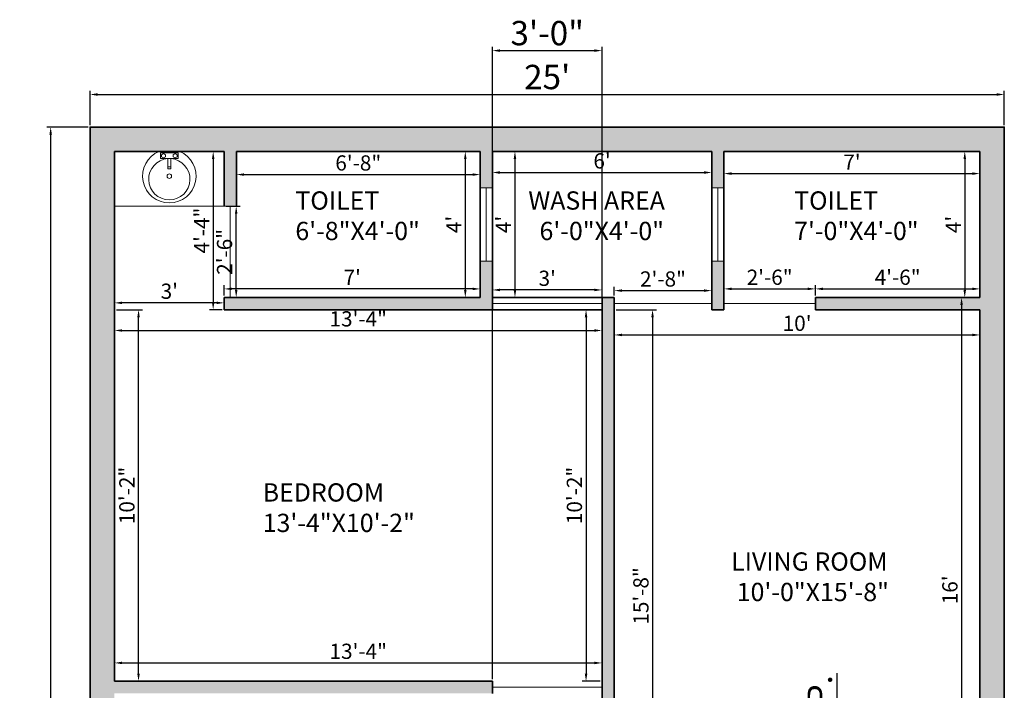
# Model space of a CAD drawing. Units: inches. Extents: x 3259 to 4981, y 1402 to 2026.
# Tile 9 of 11: x 4265 to 4588, y 1722 to 1942. Entities that reach past the tile are written whole.
import ezdxf

# ---------------------------------------------------------------- set-up
doc = ezdxf.new("R2010")
doc.units = ezdxf.units.IN
for name, color, linetype, lineweight in [('A-ANNO-DIMS', 2, 'Continuous', 13), ('A-AREA-IDEN', 7, 'Continuous', 18), ('A-DOOR', 3, 'Continuous', 18), ('A-FLOR-CASE', 8, 'Continuous', 18), ('A-FLOR-FIXT', 9, 'Continuous', 18), ('A-GLAZ', 4, 'Continuous', 18), ('A-WALL', 7, 'Continuous', 35), ('A-WALL-PATT', 252, 'Continuous', 13)]:
    doc.layers.add(name, color=color, linetype=linetype, lineweight=lineweight)
doc.styles.get("Standard").update_dxf_attribs({"font": 'arial.ttf'})
doc.dimstyles.new('ISO-25', dxfattribs={"dimtxt": 8, "dimasz": 2.5, "dimexe": 1.25, "dimexo": 0.625, "dimtad": 1, "dimdec": 1, "dimlunit": 3, "dimtxsty": 'Standard', "dimcen": 2.5, "dimclrd": 4, "dimclre": 4, "dimclrt": 1, "dimadec": 0, "dimazin": 0, "dimtfac": 1, "dimtdec": 1, "dimtmove": 0, "dimatfit": 3, "dimfxl": 1, "dimarcsym": 0})

# ---------------------------------------------------------------- blocks, each defined once
blk = doc.blocks.new('M_BATH_BASIN_Basin - Oval_P')
at = {"color": 0, "linetype": 'ByBlock', "lineweight": -2}
blk.add_lwpolyline([(0, 89.5, -5.027337), (0, -89.5)], format="xyb", close=True, dxfattribs=at)
blk.add_lwpolyline([(63.2, 12, -30), (63.2, -12, -1.097889)], format="xyb", dxfattribs=at)
for points in [[(13.2, -76.2), (13.2, 76.2), (63.2, 76.2), (63.2, -76.2)], [(19.1, 50.8), (28.7, 67.3), (47.7, 67.3), (57.2, 50.8), (47.7, 34.3), (28.7, 34.3)]]:
    blk.add_lwpolyline(points, close=True, dxfattribs=at)
for points in [[(63.2, 12), (151.6, 12), (151.6, -12), (63.2, -12)], [(134.3, 12), (134.3, -12)], [(28.7, -34.3), (47.7, -34.3), (57.2, -50.8), (47.7, -67.3), (28.7, -67.3), (19.1, -50.8), (28.7, -34.3)]]:
    blk.add_lwpolyline(points, dxfattribs=at)
blk.add_circle((216.2, 0), 20.1, dxfattribs=at)
at = {"layer": 'Defpoints'}
for p in [(0, 234), (0, -234)]:
    blk.add_point(p, dxfattribs=at)
blk = doc.blocks.new('*D83')
at = {"layer": 'A-ANNO-DIMS', "color": 0, "lineweight": -2, "transparency": 16777216}
for p, q in [((4288.33, 1907.74), (4288.33, 1919.06)), ((4290.83, 1917.81), (4585.83, 1917.81)), ((4588.33, 1907.74), (4588.33, 1919.06))]:
    blk.add_line(p, q, dxfattribs=at)
at = {"layer": 'A-ANNO-DIMS', "color": 0, "transparency": 16777216}
for points in [[(4290.83, 1918.23), (4290.83, 1917.39), (4288.33, 1917.81)], [(4585.83, 1918.23), (4585.83, 1917.39), (4588.33, 1917.81)]]:
    blk.add_solid(points, dxfattribs=at)
at = {"layer": 'Defpoints', "color": 0, "transparency": 16777216}
for p in [(4588.33, 1917.81), (4288.33, 1907.12), (4588.33, 1907.12)]:
    blk.add_point(p, dxfattribs=at)
at = {"layer": 'A-ANNO-DIMS', "color": 0, "transparency": 16777216, "insert": (4438.33, 1922.52), "char_height": 8, "attachment_point": 5}
blk.add_mtext("25'", dxfattribs=at)
blk = doc.blocks.new('*D84')
at = {"layer": 'A-ANNO-DIMS', "color": 0, "lineweight": -2, "transparency": 16777216}
for p, q in [((4287.71, 1907.12), (4274.14, 1907.12)), ((4275.39, 1904.62), (4275.39, 1477.62)), ((4287.71, 1475.12), (4274.14, 1475.12))]:
    blk.add_line(p, q, dxfattribs=at)
at = {"layer": 'A-ANNO-DIMS', "color": 0, "transparency": 16777216}
for points in [[(4274.97, 1904.62), (4275.81, 1904.62), (4275.39, 1907.12)], [(4274.97, 1477.62), (4275.81, 1477.62), (4275.39, 1475.12)]]:
    blk.add_solid(points, dxfattribs=at)
at = {"layer": 'Defpoints', "color": 0, "transparency": 16777216}
for p in [(4288.33, 1907.12), (4275.39, 1475.12), (4288.33, 1475.12)]:
    blk.add_point(p, dxfattribs=at)
at = {"layer": 'A-ANNO-DIMS', "color": 0, "transparency": 16777216, "insert": (4270.68, 1691.12), "char_height": 8, "attachment_point": 5, "rotation": 90}
blk.add_mtext("36'", dxfattribs=at)
blk = doc.blocks.new('*D79')
at = {"layer": 'A-ANNO-DIMS', "color": 0, "lineweight": -2, "transparency": 16777216}
for p, q in [((4580.33, 1846.49), (4580.33, 1837.58)), ((4460.33, 1843.37), (4460.33, 1837.58)), ((4462.83, 1838.83), (4577.83, 1838.83))]:
    blk.add_line(p, q, dxfattribs=at)
at = {"layer": 'A-ANNO-DIMS', "color": 0, "transparency": 16777216}
for points in [[(4462.83, 1839.25), (4462.83, 1838.42), (4460.33, 1838.83)], [(4577.83, 1839.25), (4577.83, 1838.42), (4580.33, 1838.83)]]:
    blk.add_solid(points, dxfattribs=at)
at = {"layer": 'Defpoints', "color": 0, "transparency": 16777216}
for p in [(4580.33, 1847.12), (4460.33, 1844), (4580.33, 1838.83)]:
    blk.add_point(p, dxfattribs=at)
at = {"layer": 'A-ANNO-DIMS', "color": 0, "transparency": 16777216, "insert": (4520.33, 1842.01), "char_height": 5, "attachment_point": 5}
blk.add_mtext("10'", dxfattribs=at)
blk = doc.blocks.new('*D80')
at = {"layer": 'A-ANNO-DIMS', "color": 0, "lineweight": -2, "transparency": 16777216}
for p, q in [((4460.96, 1847.12), (4474.15, 1847.12)), ((4472.9, 1844.62), (4472.9, 1661.62)), ((4460.96, 1659.12), (4474.15, 1659.12))]:
    blk.add_line(p, q, dxfattribs=at)
at = {"layer": 'A-ANNO-DIMS', "color": 0, "transparency": 16777216}
for points in [[(4472.49, 1844.62), (4473.32, 1844.62), (4472.9, 1847.12)], [(4472.49, 1661.62), (4473.32, 1661.62), (4472.9, 1659.12)]]:
    blk.add_solid(points, dxfattribs=at)
at = {"layer": 'Defpoints', "color": 0, "transparency": 16777216}
for p in [(4460.33, 1847.12), (4460.33, 1659.12), (4472.9, 1659.12)]:
    blk.add_point(p, dxfattribs=at)
at = {"layer": 'A-ANNO-DIMS', "color": 0, "transparency": 16777216, "insert": (4469.73, 1753.12), "char_height": 5, "attachment_point": 5, "rotation": 90}
blk.add_mtext('15\'-8"', dxfattribs=at)
blk = doc.blocks.new('*D65')
at = {"layer": 'A-ANNO-DIMS', "color": 0, "lineweight": -2, "transparency": 16777216}
for p, q in [((4336.33, 1898.49), (4336.33, 1890.25)), ((4416.33, 1898.49), (4416.33, 1890.25)), ((4338.83, 1891.5), (4413.83, 1891.5))]:
    blk.add_line(p, q, dxfattribs=at)
at = {"layer": 'A-ANNO-DIMS', "color": 0, "transparency": 16777216}
for points in [[(4338.83, 1891.92), (4338.83, 1891.09), (4336.33, 1891.5)], [(4413.83, 1891.92), (4413.83, 1891.09), (4416.33, 1891.5)]]:
    blk.add_solid(points, dxfattribs=at)
at = {"layer": 'Defpoints', "color": 0, "transparency": 16777216}
for p in [(4336.33, 1899.12), (4416.33, 1899.12), (4416.33, 1891.5)]:
    blk.add_point(p, dxfattribs=at)
at = {"layer": 'A-ANNO-DIMS', "color": 0, "transparency": 16777216, "insert": (4376.33, 1894.68), "char_height": 5, "attachment_point": 5}
blk.add_mtext('6\'-8"', dxfattribs=at)
blk = doc.blocks.new('*D66')
at = {"layer": 'A-ANNO-DIMS', "color": 0, "lineweight": -2, "transparency": 16777216}
for p, q in [((4415.71, 1899.12), (4410.21, 1899.12)), ((4411.46, 1896.62), (4411.46, 1853.62)), ((4415.71, 1851.12), (4410.21, 1851.12))]:
    blk.add_line(p, q, dxfattribs=at)
at = {"layer": 'A-ANNO-DIMS', "color": 0, "transparency": 16777216}
for points in [[(4411.04, 1896.62), (4411.87, 1896.62), (4411.46, 1899.12)], [(4411.04, 1853.62), (4411.87, 1853.62), (4411.46, 1851.12)]]:
    blk.add_solid(points, dxfattribs=at)
at = {"layer": 'Defpoints', "color": 0, "transparency": 16777216}
for p in [(4416.33, 1899.12), (4411.46, 1851.12), (4416.33, 1851.12)]:
    blk.add_point(p, dxfattribs=at)
at = {"layer": 'A-ANNO-DIMS', "color": 0, "transparency": 16777216, "insert": (4408.33, 1875.12), "char_height": 5, "attachment_point": 5, "rotation": 90}
blk.add_mtext("4'", dxfattribs=at)
blk = doc.blocks.new('*D67')
at = {"layer": 'A-ANNO-DIMS', "color": 0, "lineweight": -2, "transparency": 16777216}
for p, q in [((4420.33, 1898.49), (4420.33, 1890.93)), ((4492.33, 1898.49), (4492.33, 1890.93)), ((4422.83, 1892.18), (4489.83, 1892.18))]:
    blk.add_line(p, q, dxfattribs=at)
at = {"layer": 'A-ANNO-DIMS', "color": 0, "transparency": 16777216}
for points in [[(4422.83, 1892.6), (4422.83, 1891.76), (4420.33, 1892.18)], [(4489.83, 1892.6), (4489.83, 1891.76), (4492.33, 1892.18)]]:
    blk.add_solid(points, dxfattribs=at)
at = {"layer": 'Defpoints', "color": 0, "transparency": 16777216}
for p in [(4420.33, 1899.12), (4492.33, 1899.12), (4492.33, 1892.18)]:
    blk.add_point(p, dxfattribs=at)
at = {"layer": 'A-ANNO-DIMS', "color": 0, "transparency": 16777216, "insert": (4456.33, 1895.36), "char_height": 5, "attachment_point": 5}
blk.add_mtext("6'", dxfattribs=at)
blk = doc.blocks.new('*D68')
at = {"layer": 'A-ANNO-DIMS', "color": 0, "lineweight": -2, "transparency": 16777216}
for p, q in [((4420.96, 1899.12), (4429, 1899.12)), ((4427.75, 1896.62), (4427.75, 1853.62)), ((4420.96, 1851.12), (4429, 1851.12))]:
    blk.add_line(p, q, dxfattribs=at)
at = {"layer": 'A-ANNO-DIMS', "color": 0, "transparency": 16777216}
for points in [[(4427.33, 1896.62), (4428.16, 1896.62), (4427.75, 1899.12)], [(4427.33, 1853.62), (4428.16, 1853.62), (4427.75, 1851.12)]]:
    blk.add_solid(points, dxfattribs=at)
at = {"layer": 'Defpoints', "color": 0, "transparency": 16777216}
for p in [(4420.33, 1899.12), (4420.33, 1851.12), (4427.75, 1851.12)]:
    blk.add_point(p, dxfattribs=at)
at = {"layer": 'A-ANNO-DIMS', "color": 0, "transparency": 16777216, "insert": (4424.62, 1875.12), "char_height": 5, "attachment_point": 5, "rotation": 90}
blk.add_mtext("4'", dxfattribs=at)
blk = doc.blocks.new('*D69')
at = {"layer": 'A-ANNO-DIMS', "color": 0, "lineweight": -2, "transparency": 16777216}
for p, q in [((4496.33, 1898.49), (4496.33, 1890.58)), ((4580.33, 1898.49), (4580.33, 1890.58)), ((4498.83, 1891.83), (4577.83, 1891.83))]:
    blk.add_line(p, q, dxfattribs=at)
at = {"layer": 'A-ANNO-DIMS', "color": 0, "transparency": 16777216}
for points in [[(4498.83, 1892.25), (4498.83, 1891.41), (4496.33, 1891.83)], [(4577.83, 1892.25), (4577.83, 1891.41), (4580.33, 1891.83)]]:
    blk.add_solid(points, dxfattribs=at)
at = {"layer": 'Defpoints', "color": 0, "transparency": 16777216}
for p in [(4496.33, 1899.12), (4580.33, 1899.12), (4580.33, 1891.83)]:
    blk.add_point(p, dxfattribs=at)
at = {"layer": 'A-ANNO-DIMS', "color": 0, "transparency": 16777216, "insert": (4538.33, 1894.95), "char_height": 5, "attachment_point": 5}
blk.add_mtext("7'", dxfattribs=at)
blk = doc.blocks.new('*D70')
at = {"layer": 'A-ANNO-DIMS', "color": 0, "lineweight": -2, "transparency": 16777216}
for p, q in [((4579.71, 1899.12), (4574.11, 1899.12)), ((4575.36, 1896.62), (4575.36, 1853.62)), ((4579.71, 1851.12), (4574.11, 1851.12))]:
    blk.add_line(p, q, dxfattribs=at)
at = {"layer": 'A-ANNO-DIMS', "color": 0, "transparency": 16777216}
for points in [[(4574.94, 1896.62), (4575.77, 1896.62), (4575.36, 1899.12)], [(4574.94, 1853.62), (4575.77, 1853.62), (4575.36, 1851.12)]]:
    blk.add_solid(points, dxfattribs=at)
at = {"layer": 'Defpoints', "color": 0, "transparency": 16777216}
for p in [(4580.33, 1899.12), (4575.36, 1851.12), (4580.33, 1851.12)]:
    blk.add_point(p, dxfattribs=at)
at = {"layer": 'A-ANNO-DIMS', "color": 0, "transparency": 16777216, "insert": (4572.23, 1875.12), "char_height": 5, "attachment_point": 5, "rotation": 90}
blk.add_mtext("4'", dxfattribs=at)
blk = doc.blocks.new('*D109')
at = {"layer": 'A-ANNO-DIMS', "color": 0, "lineweight": -2, "transparency": 16777216}
for p, q in [((4331.71, 1899.12), (4327.47, 1899.12)), ((4328.72, 1896.62), (4328.72, 1849.62)), ((4331.71, 1847.12), (4327.47, 1847.12))]:
    blk.add_line(p, q, dxfattribs=at)
at = {"layer": 'A-ANNO-DIMS', "color": 0, "transparency": 16777216}
for points in [[(4328.31, 1896.62), (4329.14, 1896.62), (4328.72, 1899.12)], [(4328.31, 1849.62), (4329.14, 1849.62), (4328.72, 1847.12)]]:
    blk.add_solid(points, dxfattribs=at)
at = {"layer": 'Defpoints', "color": 0, "transparency": 16777216}
for p in [(4332.33, 1899.12), (4328.72, 1847.12), (4332.33, 1847.12)]:
    blk.add_point(p, dxfattribs=at)
at = {"layer": 'A-ANNO-DIMS', "color": 0, "transparency": 16777216, "insert": (4325.6, 1873.12), "char_height": 5, "attachment_point": 5, "rotation": 90}
blk.add_mtext('4\'-4"', dxfattribs=at)
blk = doc.blocks.new('*D110')
at = {"layer": 'A-ANNO-DIMS', "color": 0, "lineweight": -2, "transparency": 16777216}
for p, q in [((4296.33, 1847.74), (4296.33, 1850.62)), ((4329.83, 1849.37), (4298.83, 1849.37)), ((4332.33, 1847.74), (4332.33, 1850.62))]:
    blk.add_line(p, q, dxfattribs=at)
at = {"layer": 'A-ANNO-DIMS', "color": 0, "transparency": 16777216}
for points in [[(4298.83, 1849.78), (4298.83, 1848.95), (4296.33, 1849.37)], [(4329.83, 1849.78), (4329.83, 1848.95), (4332.33, 1849.37)]]:
    blk.add_solid(points, dxfattribs=at)
at = {"layer": 'Defpoints', "color": 0, "transparency": 16777216}
for p in [(4296.33, 1849.37), (4296.33, 1847.12), (4332.33, 1847.12)]:
    blk.add_point(p, dxfattribs=at)
at = {"layer": 'A-ANNO-DIMS', "color": 0, "transparency": 16777216, "insert": (4314.33, 1852.55), "char_height": 5, "attachment_point": 5}
blk.add_mtext("3'", dxfattribs=at)
blk = doc.blocks.new('*D111')
at = {"layer": 'A-ANNO-DIMS', "color": 0, "lineweight": -2, "transparency": 16777216}
for p, q in [((4296.33, 1843.44), (4296.33, 1839.05)), ((4456.33, 1843.44), (4456.33, 1839.05)), ((4298.83, 1840.3), (4453.83, 1840.3))]:
    blk.add_line(p, q, dxfattribs=at)
at = {"layer": 'A-ANNO-DIMS', "color": 0, "transparency": 16777216}
for points in [[(4298.83, 1840.71), (4298.83, 1839.88), (4296.33, 1840.3)], [(4453.83, 1840.71), (4453.83, 1839.88), (4456.33, 1840.3)]]:
    blk.add_solid(points, dxfattribs=at)
at = {"layer": 'Defpoints', "color": 0, "transparency": 16777216}
for p in [(4296.33, 1844.07), (4456.33, 1844.07), (4456.33, 1840.3)]:
    blk.add_point(p, dxfattribs=at)
at = {"layer": 'A-ANNO-DIMS', "color": 0, "transparency": 16777216, "insert": (4376.33, 1843.48), "char_height": 5, "attachment_point": 5}
blk.add_mtext('13\'-4"', dxfattribs=at)
blk = doc.blocks.new('*D112')
at = {"layer": 'A-ANNO-DIMS', "color": 0, "lineweight": -2, "transparency": 16777216}
for p, q in [((4296.96, 1847.12), (4305.48, 1847.12)), ((4304.23, 1727.62), (4304.23, 1844.62)), ((4296.96, 1725.12), (4305.48, 1725.12))]:
    blk.add_line(p, q, dxfattribs=at)
at = {"layer": 'A-ANNO-DIMS', "color": 0, "transparency": 16777216}
for points in [[(4303.81, 1844.62), (4304.64, 1844.62), (4304.23, 1847.12)], [(4303.81, 1727.62), (4304.64, 1727.62), (4304.23, 1725.12)]]:
    blk.add_solid(points, dxfattribs=at)
at = {"layer": 'Defpoints', "color": 0, "transparency": 16777216}
for p in [(4296.33, 1847.12), (4304.23, 1847.12), (4296.33, 1725.12)]:
    blk.add_point(p, dxfattribs=at)
at = {"layer": 'A-ANNO-DIMS', "color": 0, "transparency": 16777216, "insert": (4301.05, 1786.12), "char_height": 5, "attachment_point": 5, "rotation": 90}
blk.add_mtext('10\'-2"', dxfattribs=at)
blk = doc.blocks.new('*D113')
at = {"layer": 'A-ANNO-DIMS', "color": 0, "lineweight": -2, "transparency": 16777216}
for p, q in [((4296.33, 1725.74), (4296.33, 1732.36)), ((4456.33, 1725.74), (4456.33, 1732.36)), ((4298.83, 1731.11), (4453.83, 1731.11))]:
    blk.add_line(p, q, dxfattribs=at)
at = {"layer": 'A-ANNO-DIMS', "color": 0, "transparency": 16777216}
for points in [[(4298.83, 1731.53), (4298.83, 1730.7), (4296.33, 1731.11)], [(4453.83, 1731.53), (4453.83, 1730.7), (4456.33, 1731.11)]]:
    blk.add_solid(points, dxfattribs=at)
at = {"layer": 'Defpoints', "color": 0, "transparency": 16777216}
for p in [(4456.33, 1731.11), (4296.33, 1725.12), (4456.33, 1725.12)]:
    blk.add_point(p, dxfattribs=at)
at = {"layer": 'A-ANNO-DIMS', "color": 0, "transparency": 16777216, "insert": (4376.33, 1734.29), "char_height": 5, "attachment_point": 5}
blk.add_mtext('13\'-4"', dxfattribs=at)
blk = doc.blocks.new('*D114')
at = {"layer": 'A-ANNO-DIMS', "color": 0, "lineweight": -2, "transparency": 16777216}
for p, q in [((4455.71, 1847.12), (4449.83, 1847.12)), ((4451.08, 1844.62), (4451.08, 1727.62)), ((4455.71, 1725.12), (4449.83, 1725.12))]:
    blk.add_line(p, q, dxfattribs=at)
at = {"layer": 'A-ANNO-DIMS', "color": 0, "transparency": 16777216}
for points in [[(4450.66, 1844.62), (4451.5, 1844.62), (4451.08, 1847.12)], [(4450.66, 1727.62), (4451.5, 1727.62), (4451.08, 1725.12)]]:
    blk.add_solid(points, dxfattribs=at)
at = {"layer": 'Defpoints', "color": 0, "transparency": 16777216}
for p in [(4456.33, 1847.12), (4451.08, 1725.12), (4456.33, 1725.12)]:
    blk.add_point(p, dxfattribs=at)
at = {"layer": 'A-ANNO-DIMS', "color": 0, "transparency": 16777216, "insert": (4447.9, 1786.12), "char_height": 5, "attachment_point": 5, "rotation": 90}
blk.add_mtext('10\'-2"', dxfattribs=at)
blk = doc.blocks.new('*D115')
at = {"layer": 'A-ANNO-DIMS', "color": 0, "lineweight": -2, "transparency": 16777216}
for p, q in [((4579.71, 1851.12), (4573.06, 1851.12)), ((4574.31, 1848.62), (4574.31, 1661.62)), ((4579.71, 1659.12), (4573.06, 1659.12))]:
    blk.add_line(p, q, dxfattribs=at)
at = {"layer": 'A-ANNO-DIMS', "color": 0, "transparency": 16777216}
for points in [[(4573.9, 1848.62), (4574.73, 1848.62), (4574.31, 1851.12)], [(4573.9, 1661.62), (4574.73, 1661.62), (4574.31, 1659.12)]]:
    blk.add_solid(points, dxfattribs=at)
at = {"layer": 'Defpoints', "color": 0, "transparency": 16777216}
for p in [(4580.33, 1851.12), (4574.31, 1659.12), (4580.33, 1659.12)]:
    blk.add_point(p, dxfattribs=at)
at = {"layer": 'A-ANNO-DIMS', "color": 0, "transparency": 16777216, "insert": (4571.13, 1755.12), "char_height": 5, "attachment_point": 5, "rotation": 90}
blk.add_mtext("16'", dxfattribs=at)
blk = doc.blocks.new('*D121')
at = {"layer": 'A-ANNO-DIMS', "color": 0, "lineweight": -2, "transparency": 16777216}
for p, q in [((4332.33, 1851.74), (4332.33, 1855.2)), ((4416.33, 1851.74), (4416.33, 1855.2)), ((4413.83, 1853.95), (4334.83, 1853.95))]:
    blk.add_line(p, q, dxfattribs=at)
at = {"layer": 'A-ANNO-DIMS', "color": 0, "transparency": 16777216}
for points in [[(4334.83, 1854.37), (4334.83, 1853.54), (4332.33, 1853.95)], [(4413.83, 1854.37), (4413.83, 1853.54), (4416.33, 1853.95)]]:
    blk.add_solid(points, dxfattribs=at)
at = {"layer": 'Defpoints', "color": 0, "transparency": 16777216}
for p in [(4332.33, 1853.95), (4332.33, 1851.12), (4416.33, 1851.12)]:
    blk.add_point(p, dxfattribs=at)
at = {"layer": 'A-ANNO-DIMS', "color": 0, "transparency": 16777216, "insert": (4374.33, 1857.08), "char_height": 5, "attachment_point": 5}
blk.add_mtext("7'", dxfattribs=at)
blk = doc.blocks.new('*D122')
at = {"layer": 'A-ANNO-DIMS', "color": 0, "lineweight": -2, "transparency": 16777216}
for p, q in [((4332.96, 1881.12), (4337.53, 1881.12)), ((4336.28, 1853.62), (4336.28, 1878.62)), ((4332.96, 1851.12), (4337.53, 1851.12))]:
    blk.add_line(p, q, dxfattribs=at)
at = {"layer": 'A-ANNO-DIMS', "color": 0, "transparency": 16777216}
for points in [[(4335.86, 1878.62), (4336.69, 1878.62), (4336.28, 1881.12)], [(4335.86, 1853.62), (4336.69, 1853.62), (4336.28, 1851.12)]]:
    blk.add_solid(points, dxfattribs=at)
at = {"layer": 'Defpoints', "color": 0, "transparency": 16777216}
for p in [(4332.33, 1881.12), (4336.28, 1881.12), (4332.33, 1851.12)]:
    blk.add_point(p, dxfattribs=at)
at = {"layer": 'A-ANNO-DIMS', "color": 0, "transparency": 16777216, "insert": (4333.1, 1866.12), "char_height": 5, "attachment_point": 5, "rotation": 90}
blk.add_mtext('2\'-6"', dxfattribs=at)
blk = doc.blocks.new('*D123')
at = {"layer": 'A-ANNO-DIMS', "color": 0, "lineweight": -2, "transparency": 16777216}
for p, q in [((4420.33, 1847.74), (4420.33, 1854.87)), ((4456.33, 1847.74), (4456.33, 1854.87)), ((4453.83, 1853.62), (4422.83, 1853.62))]:
    blk.add_line(p, q, dxfattribs=at)
at = {"layer": 'A-ANNO-DIMS', "color": 0, "transparency": 16777216}
for points in [[(4422.83, 1854.03), (4422.83, 1853.2), (4420.33, 1853.62)], [(4453.83, 1854.03), (4453.83, 1853.2), (4456.33, 1853.62)]]:
    blk.add_solid(points, dxfattribs=at)
at = {"layer": 'Defpoints', "color": 0, "transparency": 16777216}
for p in [(4420.33, 1853.62), (4420.33, 1847.12), (4456.33, 1847.12)]:
    blk.add_point(p, dxfattribs=at)
at = {"layer": 'A-ANNO-DIMS', "color": 0, "transparency": 16777216, "insert": (4438.33, 1856.8), "char_height": 5, "attachment_point": 5}
blk.add_mtext("3'", dxfattribs=at)
blk = doc.blocks.new('*D124')
at = {"layer": 'A-ANNO-DIMS', "color": 0, "lineweight": -2, "transparency": 16777216}
for p, q in [((4460.33, 1851.74), (4460.33, 1854.64)), ((4492.33, 1851.74), (4492.33, 1854.64)), ((4462.83, 1853.39), (4489.83, 1853.39))]:
    blk.add_line(p, q, dxfattribs=at)
at = {"layer": 'A-ANNO-DIMS', "color": 0, "transparency": 16777216}
for points in [[(4462.83, 1853.81), (4462.83, 1852.98), (4460.33, 1853.39)], [(4489.83, 1853.81), (4489.83, 1852.98), (4492.33, 1853.39)]]:
    blk.add_solid(points, dxfattribs=at)
at = {"layer": 'Defpoints', "color": 0, "transparency": 16777216}
for p in [(4492.33, 1853.39), (4460.33, 1851.12), (4492.33, 1851.12)]:
    blk.add_point(p, dxfattribs=at)
at = {"layer": 'A-ANNO-DIMS', "color": 0, "transparency": 16777216, "insert": (4476.33, 1856.57), "char_height": 5, "attachment_point": 5}
blk.add_mtext('2\'-8"', dxfattribs=at)
blk = doc.blocks.new('*D125')
at = {"layer": 'A-ANNO-DIMS', "color": 0, "lineweight": -2, "transparency": 16777216}
for p, q in [((4496.33, 1854.02), (4496.33, 1855.21)), ((4526.33, 1851.74), (4526.33, 1855.21)), ((4498.83, 1853.96), (4523.83, 1853.96))]:
    blk.add_line(p, q, dxfattribs=at)
at = {"layer": 'A-ANNO-DIMS', "color": 0, "transparency": 16777216}
for points in [[(4498.83, 1854.38), (4498.83, 1853.54), (4496.33, 1853.96)], [(4523.83, 1854.38), (4523.83, 1853.54), (4526.33, 1853.96)]]:
    blk.add_solid(points, dxfattribs=at)
at = {"layer": 'Defpoints', "color": 0, "transparency": 16777216}
for p in [(4496.33, 1853.39), (4526.33, 1853.96), (4526.33, 1851.12)]:
    blk.add_point(p, dxfattribs=at)
at = {"layer": 'A-ANNO-DIMS', "color": 0, "transparency": 16777216, "insert": (4511.33, 1857.14), "char_height": 5, "attachment_point": 5}
blk.add_mtext('2\'-6"', dxfattribs=at)
blk = doc.blocks.new('*D126')
at = {"layer": 'A-ANNO-DIMS', "color": 0, "lineweight": -2, "transparency": 16777216}
for p, q in [((4526.33, 1851.74), (4526.33, 1855.21)), ((4580.33, 1851.74), (4580.33, 1855.21)), ((4528.83, 1853.96), (4577.83, 1853.96))]:
    blk.add_line(p, q, dxfattribs=at)
at = {"layer": 'A-ANNO-DIMS', "color": 0, "transparency": 16777216}
for points in [[(4528.83, 1854.38), (4528.83, 1853.54), (4526.33, 1853.96)], [(4577.83, 1854.38), (4577.83, 1853.54), (4580.33, 1853.96)]]:
    blk.add_solid(points, dxfattribs=at)
at = {"layer": 'Defpoints', "color": 0, "transparency": 16777216}
for p in [(4580.33, 1853.96), (4526.33, 1851.12), (4580.33, 1851.12)]:
    blk.add_point(p, dxfattribs=at)
at = {"layer": 'A-ANNO-DIMS', "color": 0, "transparency": 16777216, "insert": (4553.33, 1857.14), "char_height": 5, "attachment_point": 5}
blk.add_mtext('4\'-6"', dxfattribs=at)
blk = doc.blocks.new('VENT-24x4')
for p, q in [((0, 24), (4, 24)), ((2, 24), (2, 0)), ((0, 0), (4, 0))]:
    blk.add_line(p, q)
blk = doc.blocks.new('*D171')
at = {"layer": 'A-ANNO-DIMS', "color": 4, "lineweight": -2, "transparency": 16777216}
for p, q in [((4533.53, 1675.12), (4533.53, 1727.77)), ((4526.96, 1675.12), (4534.78, 1675.12)), ((4533.53, 1653.62), (4533.53, 1672.62)), ((4526.96, 1651.12), (4534.78, 1651.12))]:
    blk.add_line(p, q, dxfattribs=at)
at = {"layer": 'A-ANNO-DIMS', "color": 4, "transparency": 16777216}
for points in [[(4533.11, 1672.62), (4533.95, 1672.62), (4533.53, 1675.12)], [(4533.11, 1653.62), (4533.95, 1653.62), (4533.53, 1651.12)]]:
    blk.add_solid(points, dxfattribs=at)
at = {"layer": 'Defpoints', "color": 0, "transparency": 16777216}
for p in [(4526.33, 1675.12), (4533.53, 1675.12), (4526.33, 1651.12)]:
    blk.add_point(p, dxfattribs=at)
at = {"layer": 'A-ANNO-DIMS', "color": 1, "transparency": 16777216, "insert": (4528.82, 1702.69), "char_height": 8, "attachment_point": 5, "rotation": 90}
blk.add_mtext('2\'-0" TYP.', dxfattribs=at)
blk = doc.blocks.new('*D195')
at = {"layer": 'A-ANNO-DIMS', "color": 4, "lineweight": -2, "transparency": 16777216}
for p, q in [((4420.33, 1725.74), (4420.33, 1933.47)), ((4422.83, 1932.22), (4453.83, 1932.22)), ((4456.33, 1723.74), (4456.33, 1933.47))]:
    blk.add_line(p, q, dxfattribs=at)
at = {"layer": 'A-ANNO-DIMS', "color": 4, "transparency": 16777216}
for points in [[(4422.83, 1932.63), (4422.83, 1931.8), (4420.33, 1932.22)], [(4453.83, 1932.63), (4453.83, 1931.8), (4456.33, 1932.22)]]:
    blk.add_solid(points, dxfattribs=at)
at = {"layer": 'Defpoints', "color": 0, "transparency": 16777216}
for p in [(4456.33, 1932.22), (4420.33, 1725.12), (4456.33, 1723.12)]:
    blk.add_point(p, dxfattribs=at)
at = {"layer": 'A-ANNO-DIMS', "color": 1, "transparency": 16777216, "insert": (4438.33, 1936.93), "char_height": 8, "attachment_point": 5}
blk.add_mtext('3\'-0"', dxfattribs=at)

msp = doc.modelspace()

# ---------------------------------------------------------------- hatches: boundary and pattern name
at = {"layer": 'A-WALL-PATT'}
h = msp.add_hatch(color=256, dxfattribs=at)
h.dxf.hatch_style = 1
h.paths.add_polyline_path([(4588.33, 1907.12), (4288.33, 1907.12), (4288.33, 1475.12), (4385.33, 1475.12), (4385.33, 1483.12), (4296.33, 1483.12), (4296.33, 1579.12), (4408.33, 1579.12), (4408.33, 1583.12), (4296.33, 1583.12), (4296.33, 1721.12), (4420.33, 1721.12), (4420.33, 1725.12), (4296.33, 1725.12), (4296.33, 1899.12), (4332.33, 1899.12), (4332.33, 1881.12), (4336.33, 1881.12), (4336.33, 1899.12), (4416.33, 1899.12), (4416.33, 1887.12), (4420.33, 1887.12), (4420.33, 1899.12), (4492.33, 1899.12), (4492.33, 1887.12), (4496.33, 1887.12), (4496.33, 1899.12), (4580.33, 1899.12), (4580.33, 1851.12), (4526.33, 1851.12), (4526.33, 1847.12), (4580.33, 1847.12), (4580.33, 1659.12), (4574.33, 1659.12), (4574.33, 1651.12), (4580.33, 1651.12), (4580.33, 1475.12), (4588.33, 1475.12)])
h.paths.add_polyline_path([(4420.33, 1863.12), (4416.33, 1863.12), (4416.33, 1851.12), (4332.33, 1851.12), (4332.33, 1847.12), (4370.16, 1847.12), (4370.16, 1847.13), (4370.21, 1847.13), (4370.21, 1847.12), (4374.23, 1847.12), (4374.23, 1847.12), (4374.28, 1847.12), (4420.33, 1847.12)], flags=17)
h.paths.add_polyline_path([(4496.33, 1863.12), (4492.33, 1863.12), (4492.33, 1847.12), (4496.33, 1847.12)], flags=17)
h.paths.add_polyline_path([(4460.33, 1851.12), (4456.33, 1851.12), (4456.33, 1715.12), (4460.33, 1715.12), (4460.33, 1777.43), (4460.32, 1777.43), (4460.32, 1777.47), (4460.33, 1777.47), (4460.33, 1781.5), (4460.33, 1781.5), (4460.33, 1781.55)], flags=17)
h.paths.add_polyline_path([(4478.33, 1659.12), (4460.33, 1659.12), (4460.33, 1667.12), (4456.33, 1667.12), (4456.33, 1483.12), (4460.33, 1483.12), (4460.33, 1651.12), (4478.33, 1651.12)], flags=17)
h.paths.add_polyline_path([(4538.33, 1659.12), (4526.33, 1659.12), (4526.33, 1651.12), (4538.33, 1651.12)], flags=17)
h.paths.add_polyline_path([(4460.33, 1483.12), (4445.33, 1483.12), (4445.33, 1475.12), (4460.33, 1475.12)], flags=17)

# ---------------------------------------------------------------- linework, layer by layer
at = {"layer": 'A-DOOR'}
for p, q in [((4334.33, 1881.12), (4334.33, 1851.12)), ((4460.33, 1849.12), (4492.33, 1849.12)), ((4526.33, 1849.12), (4496.33, 1849.12)), ((4420.33, 1723.12), (4456.33, 1723.12))]:
    msp.add_line(p, q, dxfattribs=at)
at = {"layer": 'A-FLOR-CASE'}
msp.add_line((4296.33, 1881.12), (4336.33, 1881.12), dxfattribs=at)
at = {"layer": 'A-GLAZ'}
msp.add_line((4420.33, 1849.12), (4456.33, 1849.12), dxfattribs=at)
at = {"layer": 'A-WALL'}
for p, q in [((4296.33, 1899.12), (4332.33, 1899.12)), ((4296.33, 1725.12), (4296.33, 1899.12)), ((4332.33, 1899.12), (4332.33, 1881.12)), ((4336.33, 1899.12), (4416.33, 1899.12)), ((4336.33, 1899.12), (4336.33, 1881.12)), ((4416.33, 1899.12), (4416.33, 1851.12)), ((4420.33, 1899.12), (4492.33, 1899.12)), ((4420.33, 1899.12), (4420.33, 1847.12)), ((4492.33, 1899.12), (4492.33, 1847.12)), ((4496.33, 1899.12), (4580.33, 1899.12)), ((4496.33, 1899.12), (4496.33, 1847.12)), ((4580.33, 1899.12), (4580.33, 1851.12)), ((4332.33, 1851.12), (4416.33, 1851.12)), ((4332.33, 1851.12), (4332.33, 1847.12)), ((4420.33, 1851.12), (4460.33, 1851.12)), ((4456.33, 1713.12), (4456.33, 1851.12)), ((4460.33, 1713.12), (4460.33, 1851.12)), ((4526.33, 1851.12), (4580.33, 1851.12)), ((4526.33, 1851.12), (4526.33, 1847.12)), ((4332.33, 1847.12), (4456.33, 1847.12)), ((4492.33, 1847.12), (4496.33, 1847.12)), ((4526.33, 1847.12), (4580.33, 1847.12)), ((4580.33, 1847.12), (4580.33, 1659.12)), ((4296.33, 1725.12), (4420.33, 1725.12)), ((4420.33, 1721.12), (4420.33, 1725.12))]:
    msp.add_line(p, q, dxfattribs=at)
msp.add_lwpolyline([(4460.33, 1475.12), (4288.33, 1475.12), (4288.33, 1907.12), (4588.33, 1907.12), (4588.33, 1475.12), (4580.33, 1475.12)], dxfattribs=at)

# ---------------------------------------------------------------- block references
at = {"layer": 'A-FLOR-FIXT', "xscale": -0.0376189459335944, "yscale": 0.0376189459335944, "zscale": 0.0376189459335944, "rotation": 90}
msp.add_blockref('M_BATH_BASIN_Basin - Oval_P', (4314.33, 1899.12), dxfattribs=at)
at = {"layer": 'A-GLAZ'}
msp.add_blockref('VENT-24x4', (4416.33, 1863.12), dxfattribs=at)
at = {"layer": 'A-GLAZ', "rotation": 180}
msp.add_blockref('VENT-24x4', (4496.33, 1887.12), dxfattribs=at)

# ---------------------------------------------------------------- texts
at = {"layer": 'A-AREA-IDEN', "char_height": 6, "attachment_point": 1}
for s, width, insert in [('TOILET\\P6\'-8"X4\'-0"', 127.3061, (4355.69, 1885.99)), ('WASH AREA\\P  6\'-0"X4\'-0"', 127.3061, (4432.14, 1885.99)), ('TOILET\\P7\'-0"X4\'-0"', 127.3061, (4519.35, 1885.99)), ('BEDROOM\\P13\'-4"X10\'-2"', 86.9528, (4344.97, 1790.11)), ('LIVING ROOM\\P 10\'-0"X15\'-8"', 127.3061, (4498.69, 1767.42))]:
    msp.add_mtext_dynamic_manual_height_columns(s, width=width, gutter_width=12.5, heights=[0], dxfattribs=dict(at, insert=insert))

# ---------------------------------------------------------------- dimensions: what is measured, and where the dimension line sits
at = {"layer": 'A-ANNO-DIMS'}
for base, p1, p2, override, picture, middle in [((4456.33, 1932.22), (4420.33, 1725.12), (4456.33, 1723.12), {"dimdec": 1, "dimlfac": 1, "dimrnd": 0, "dimzin": 1, "dimdsep": 46, "dimlunit": 4, "dimfrac": 2}, '*D195', (4438.33, 1936.93)), ((4588.33, 1917.81), (4288.33, 1907.12), (4588.33, 1907.12), {"dimclrd": 0, "dimclre": 0, "dimclrt": 0}, '*D83', (4438.33, 1922.52)), ((4416.33, 1891.5), (4336.33, 1899.12), (4416.33, 1899.12), {"dimtxt": 5, "dimclrd": 0, "dimclre": 0, "dimclrt": 0}, '*D65', (4376.33, 1894.68)), ((4492.33, 1892.18), (4420.33, 1899.12), (4492.33, 1899.12), {"dimtxt": 5, "dimclrd": 0, "dimclre": 0, "dimclrt": 0}, '*D67', (4456.33, 1895.36)), ((4580.33, 1891.83), (4496.33, 1899.12), (4580.33, 1899.12), {"dimtxt": 5, "dimclrd": 0, "dimclre": 0, "dimclrt": 0}, '*D69', (4538.33, 1894.95)), ((4332.33, 1853.95), (4416.33, 1851.12), (4332.33, 1851.12), {"dimtxt": 5, "dimclrd": 0, "dimclre": 0, "dimclrt": 0}, '*D121', (4374.33, 1857.08)), ((4420.33, 1853.62), (4456.33, 1847.12), (4420.33, 1847.12), {"dimtxt": 5, "dimclrd": 0, "dimclre": 0, "dimclrt": 0}, '*D123', (4438.33, 1856.8)), ((4492.33, 1853.39), (4460.33, 1851.12), (4492.33, 1851.12), {"dimtxt": 5, "dimclrd": 0, "dimclre": 0, "dimclrt": 0}, '*D124', (4476.33, 1856.57)), ((4526.33, 1853.96), (4496.33, 1853.39), (4526.33, 1851.12), {"dimtxt": 5, "dimclrd": 0, "dimclre": 0, "dimclrt": 0}, '*D125', (4511.33, 1857.14)), ((4580.33, 1853.96), (4526.33, 1851.12), (4580.33, 1851.12), {"dimtxt": 5, "dimclrd": 0, "dimclre": 0, "dimclrt": 0, "dimtmove": 1}, '*D126', (4553.33, 1857.14)), ((4296.33, 1849.37), (4332.33, 1847.12), (4296.33, 1847.12), {"dimtxt": 5, "dimclrd": 0, "dimclre": 0, "dimclrt": 0}, '*D110', (4314.33, 1852.55)), ((4456.33, 1840.3), (4296.33, 1844.07), (4456.33, 1844.07), {"dimtxt": 5, "dimclrd": 0, "dimclre": 0, "dimclrt": 0}, '*D111', (4376.33, 1843.48)), ((4580.33, 1838.83), (4460.33, 1844), (4580.33, 1847.12), {"dimtxt": 5, "dimclrd": 0, "dimclre": 0, "dimclrt": 0}, '*D79', (4520.33, 1842.01)), ((4456.33, 1731.11), (4296.33, 1725.12), (4456.33, 1725.12), {"dimtxt": 5, "dimclrd": 0, "dimclre": 0, "dimclrt": 0}, '*D113', (4376.33, 1734.29))]:
    dim = msp.add_linear_dim(base=base, p1=p1, p2=p2, dimstyle='ISO-25', override=override, dxfattribs=at)
    dim.commit()
    dim.dimension.update_dxf_attribs({"geometry": picture, "text_midpoint": middle})
for base, p1, p2, override, picture, middle in [((4275.39, 1475.12), (4288.33, 1907.12), (4288.33, 1475.12), {"dimclrd": 0, "dimclre": 0, "dimclrt": 0}, '*D84', (4270.68, 1691.12)), ((4328.72, 1847.12), (4332.33, 1899.12), (4332.33, 1847.12), {"dimtxt": 5, "dimclrd": 0, "dimclre": 0, "dimclrt": 0}, '*D109', (4325.6, 1873.12)), ((4411.46, 1851.12), (4416.33, 1899.12), (4416.33, 1851.12), {"dimtxt": 5, "dimclrd": 0, "dimclre": 0, "dimclrt": 0}, '*D66', (4408.33, 1875.12)), ((4427.75, 1851.12), (4420.33, 1899.12), (4420.33, 1851.12), {"dimtxt": 5, "dimclrd": 0, "dimclre": 0, "dimclrt": 0}, '*D68', (4424.62, 1875.12)), ((4575.36, 1851.12), (4580.33, 1899.12), (4580.33, 1851.12), {"dimtxt": 5, "dimclrd": 0, "dimclre": 0, "dimclrt": 0}, '*D70', (4572.23, 1875.12)), ((4336.28, 1881.12), (4332.33, 1851.12), (4332.33, 1881.12), {"dimtxt": 5, "dimclrd": 0, "dimclre": 0, "dimclrt": 0}, '*D122', (4333.1, 1866.12)), ((4574.31, 1659.12), (4580.33, 1851.12), (4580.33, 1659.12), {"dimtxt": 5, "dimclrd": 0, "dimclre": 0, "dimclrt": 0}, '*D115', (4571.13, 1755.12)), ((4304.23, 1847.12), (4296.33, 1725.12), (4296.33, 1847.12), {"dimtxt": 5, "dimclrd": 0, "dimclre": 0, "dimclrt": 0}, '*D112', (4301.05, 1786.12)), ((4451.08, 1725.12), (4456.33, 1847.12), (4456.33, 1725.12), {"dimtxt": 5, "dimclrd": 0, "dimclre": 0, "dimclrt": 0}, '*D114', (4447.9, 1786.12)), ((4472.9, 1659.12), (4460.33, 1847.12), (4460.33, 1659.12), {"dimtxt": 5, "dimclrd": 0, "dimclre": 0, "dimclrt": 0}, '*D80', (4469.73, 1753.12))]:
    dim = msp.add_linear_dim(base=base, p1=p1, p2=p2, angle=90, dimstyle='ISO-25', override=override, dxfattribs=at)
    dim.commit()
    dim.dimension.update_dxf_attribs({"geometry": picture, "text_midpoint": middle})
dim = msp.add_linear_dim(base=(4533.53, 1675.12), p1=(4526.33, 1651.12), p2=(4526.33, 1675.12), angle=90, text='<> TYP.', dimstyle='ISO-25', override={"dimdec": 1, "dimlfac": 1, "dimrnd": 0, "dimzin": 1, "dimdsep": 46, "dimlunit": 4, "dimfrac": 2}, dxfattribs=at)
dim.commit()
dim.dimension.update_dxf_attribs({"geometry": '*D171', "text_midpoint": (4528.82, 1702.69)})

doc.saveas('drawing.dxf')
